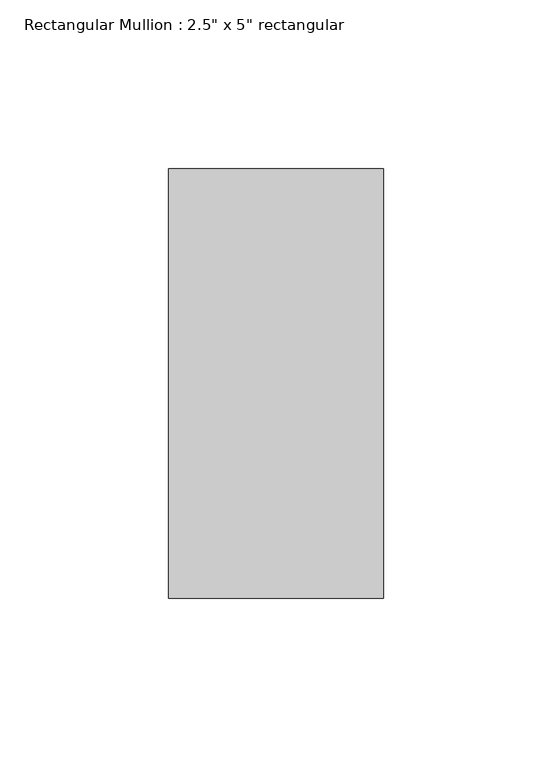
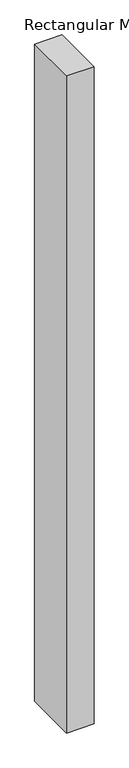
"""IFC4 building model written with IfcOpenShell, lengths in millimetres: member geometry."""

from ifc_helpers import new_model, si_unit, frame, origin, place, context, project, spatial, polyline, outline, extrude, source, transform, mapped, element, save


def member_491a8506(model_context):
    return source(origin(), model_context, "Body", "SweptSolid", [
        extrude(outline(polyline([(31.75, 63.5), (31.75, -63.5), (-31.75, -63.5), (-31.75, 63.5), (31.75, 63.5)])), frame((0.0, 0.0, -1602.5825326), z_axis=(0.0, 0.0, 1.0), x_axis=(1.0, 0.0, 0.0)), (0.0, 0.0, 1.0), 1602.5825326),
    ])


if __name__ == "__main__":
    model = new_model("IFC4")
    model_context = context("Model", 3, world=origin())
    ifc_project = project(units=[si_unit("LENGTHUNIT", "METRE", prefix="MILLI")], contexts=[model_context])
    site = spatial("IfcSite", under=ifc_project)
    building = spatial("IfcBuilding", under=site)
    placement = place(None, origin())
    member_shape = member_491a8506(model_context)
    element("IfcMember", 1, ObjectType="Rectangular Mullion : 2.5\" x 5\" rectangular", at=placement, inside=building, context=model_context, shape_type="MappedRepresentation", body=[
        mapped(member_shape, transform((0.0, 0.0, 0.0), x_axis=(1.0, 0.0, 0.0), y_axis=(0.0, 1.0, 0.0), z_axis=(0.0, 0.0, 1.0))),
    ])
    save(model, "model.ifc")

# Revit data of these elements
# Type "Rectangular Mullion : 2.5\" x 5\" rectangular"
#   built-in parameter 1007304 = 0.416667 (stored number, unit not read)
#   built-in parameter 1007301 = 0.104167 (stored number, unit not read)
#   built-in parameter 1007300 = 0.104167 (stored number, unit not read)
# Element 1 (IfcMember, "Rectangular Mullion : 2.5\" x 5\" rectangular")
#   Materials on its faces: "Aluminum"
# Materials
#   "Aluminum": class "Metal", colour RGB 247 247 247, transparency 0, Description = "Aluminum 6061", Cost = 0
